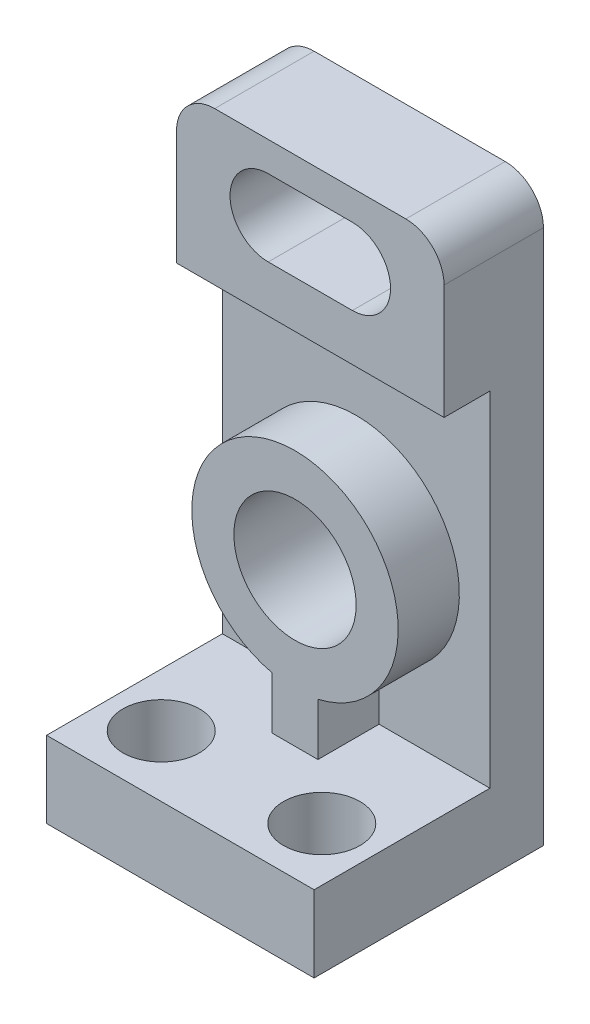
ISO-10303-21;
HEADER;
FILE_DESCRIPTION(('STEP AP214'),'2;1');
FILE_NAME('part.step','',(''),(''),'','','');
FILE_SCHEMA(('AUTOMOTIVE_DESIGN { 1 0 10303 214 1 1 1 1 }'));
ENDSEC;
DATA;
#1=APPLICATION_CONTEXT('core data for automotive mechanical design processes');
#2=APPLICATION_PROTOCOL_DEFINITION('international standard','automotive_design',2000,#1);
#3=PRODUCT_CONTEXT('',#1,'mechanical');
#4=PRODUCT('Part','Part','',(#3));
#5=PRODUCT_RELATED_PRODUCT_CATEGORY('part','',(#4));
#6=PRODUCT_DEFINITION_FORMATION('','',#4);
#7=PRODUCT_DEFINITION_CONTEXT('part definition',#1,'design');
#8=PRODUCT_DEFINITION('design','',#6,#7);
#9=PRODUCT_DEFINITION_SHAPE('','',#8);
#10=(LENGTH_UNIT() NAMED_UNIT(*) SI_UNIT(.MILLI.,.METRE.));
#11=(NAMED_UNIT(*) PLANE_ANGLE_UNIT() SI_UNIT($,.RADIAN.));
#12=(NAMED_UNIT(*) SI_UNIT($,.STERADIAN.) SOLID_ANGLE_UNIT());
#13=UNCERTAINTY_MEASURE_WITH_UNIT(LENGTH_MEASURE(1.E-05),#10,'distance_accuracy_value','');
#14=(GEOMETRIC_REPRESENTATION_CONTEXT(3) GLOBAL_UNCERTAINTY_ASSIGNED_CONTEXT((#13)) GLOBAL_UNIT_ASSIGNED_CONTEXT((#10,
#11,#12)) REPRESENTATION_CONTEXT('',''));
#15=CARTESIAN_POINT('',(0.,0.,0.));
#16=DIRECTION('',(0.,0.,1.));
#17=DIRECTION('',(1.,0.,0.));
#18=AXIS2_PLACEMENT_3D('',#15,#16,#17);
#19=CARTESIAN_POINT('',(0.,10.,0.));
#20=DIRECTION('',(0.,1.,0.));
#21=DIRECTION('',(0.,0.,1.));
#22=AXIS2_PLACEMENT_3D('',#19,#20,#21);
#23=PLANE('',#22);
#24=CARTESIAN_POINT('',(10.5,10.,7.));
#25=DIRECTION('',(0.,1.,0.));
#26=DIRECTION('',(0.,0.,1.));
#27=AXIS2_PLACEMENT_3D('',#24,#25,#26);
#28=CIRCLE('',#27,5.);
#29=CARTESIAN_POINT('',(10.5,10.,12.));
#30=VERTEX_POINT('',#29);
#31=EDGE_CURVE('E288',#30,#30,#28,.T.);
#32=ORIENTED_EDGE('',*,*,#31,.F.);
#33=EDGE_LOOP('',(#32));
#34=FACE_BOUND('',#33,.T.);
#35=CARTESIAN_POINT('',(-10.5,10.,7.));
#36=DIRECTION('',(0.,1.,0.));
#37=DIRECTION('',(0.,0.,1.));
#38=AXIS2_PLACEMENT_3D('',#35,#36,#37);
#39=CIRCLE('',#38,5.);
#40=CARTESIAN_POINT('',(-10.5,10.,12.));
#41=VERTEX_POINT('',#40);
#42=EDGE_CURVE('E619',#41,#41,#39,.T.);
#43=ORIENTED_EDGE('',*,*,#42,.F.);
#44=EDGE_LOOP('',(#43));
#45=FACE_BOUND('',#44,.T.);
#46=DIRECTION('',(1.,0.,0.));
#47=VECTOR('',#46,1.);
#48=CARTESIAN_POINT('',(-17.5,10.,-8.));
#49=LINE('',#48,#47);
#50=CARTESIAN_POINT('',(3.,10.,-8.));
#51=VERTEX_POINT('',#50);
#52=CARTESIAN_POINT('',(17.5,10.,-8.));
#53=VERTEX_POINT('',#52);
#54=EDGE_CURVE('E193',#51,#53,#49,.T.);
#55=ORIENTED_EDGE('',*,*,#54,.F.);
#56=DIRECTION('',(0.,0.,-1.));
#57=VECTOR('',#56,1.);
#58=CARTESIAN_POINT('',(3.,10.,0.));
#59=LINE('',#58,#57);
#60=CARTESIAN_POINT('',(3.,10.,0.));
#61=VERTEX_POINT('',#60);
#62=EDGE_CURVE('E172',#61,#51,#59,.T.);
#63=ORIENTED_EDGE('',*,*,#62,.F.);
#64=DIRECTION('',(1.,0.,0.));
#65=VECTOR('',#64,1.);
#66=CARTESIAN_POINT('',(-3.,10.,0.));
#67=LINE('',#66,#65);
#68=CARTESIAN_POINT('',(-3.,10.,0.));
#69=VERTEX_POINT('',#68);
#70=EDGE_CURVE('E181',#69,#61,#67,.T.);
#71=ORIENTED_EDGE('',*,*,#70,.F.);
#72=DIRECTION('',(0.,0.,-1.));
#73=VECTOR('',#72,1.);
#74=CARTESIAN_POINT('',(-3.,10.,0.));
#75=LINE('',#74,#73);
#76=CARTESIAN_POINT('',(-3.,10.,-8.));
#77=VERTEX_POINT('',#76);
#78=EDGE_CURVE('E632',#69,#77,#75,.T.);
#79=ORIENTED_EDGE('',*,*,#78,.T.);
#80=CARTESIAN_POINT('',(-17.5,10.,-8.));
#81=VERTEX_POINT('',#80);
#82=EDGE_CURVE('E252',#81,#77,#49,.T.);
#83=ORIENTED_EDGE('',*,*,#82,.F.);
#84=DIRECTION('',(0.,0.,1.));
#85=VECTOR('',#84,1.);
#86=CARTESIAN_POINT('',(-17.5,10.,-15.));
#87=LINE('',#86,#85);
#88=CARTESIAN_POINT('',(-17.5,10.,15.));
#89=VERTEX_POINT('',#88);
#90=EDGE_CURVE('E263',#81,#89,#87,.T.);
#91=ORIENTED_EDGE('',*,*,#90,.T.);
#92=DIRECTION('',(1.,0.,0.));
#93=VECTOR('',#92,1.);
#94=CARTESIAN_POINT('',(-17.5,10.,15.));
#95=LINE('',#94,#93);
#96=CARTESIAN_POINT('',(17.5,10.,15.));
#97=VERTEX_POINT('',#96);
#98=EDGE_CURVE('E264',#89,#97,#95,.T.);
#99=ORIENTED_EDGE('',*,*,#98,.T.);
#100=DIRECTION('',(0.,0.,-1.));
#101=VECTOR('',#100,1.);
#102=CARTESIAN_POINT('',(17.5,10.,-15.));
#103=LINE('',#102,#101);
#104=EDGE_CURVE('E256',#97,#53,#103,.T.);
#105=ORIENTED_EDGE('',*,*,#104,.T.);
#106=EDGE_LOOP('',(#55,#63,#71,#79,#83,#91,#99,#105));
#107=FACE_BOUND('',#106,.T.);
#108=ADVANCED_FACE('F50',(#34,#45,#107),#23,.T.);
#109=CARTESIAN_POINT('',(-17.5,75.,-8.));
#110=DIRECTION('',(0.,0.,-1.));
#111=DIRECTION('',(-1.,0.,0.));
#112=AXIS2_PLACEMENT_3D('',#109,#110,#111);
#113=PLANE('',#112);
#114=DIRECTION('',(0.,1.,0.));
#115=VECTOR('',#114,1.);
#116=CARTESIAN_POINT('',(3.,16.8375534189118,-8.));
#117=LINE('',#116,#115);
#118=CARTESIAN_POINT('',(3.,16.8375534189118,-8.));
#119=VERTEX_POINT('',#118);
#120=EDGE_CURVE('E629',#51,#119,#117,.T.);
#121=ORIENTED_EDGE('',*,*,#120,.F.);
#122=ORIENTED_EDGE('',*,*,#54,.T.);
#123=DIRECTION('',(0.,-1.,0.));
#124=VECTOR('',#123,1.);
#125=CARTESIAN_POINT('',(17.5,75.,-8.));
#126=LINE('',#125,#124);
#127=CARTESIAN_POINT('',(17.5,55.,-8.));
#128=VERTEX_POINT('',#127);
#129=EDGE_CURVE('E249',#128,#53,#126,.T.);
#130=ORIENTED_EDGE('',*,*,#129,.F.);
#131=DIRECTION('',(1.,0.,0.));
#132=VECTOR('',#131,1.);
#133=CARTESIAN_POINT('',(-17.5,55.,-8.));
#134=LINE('',#133,#132);
#135=CARTESIAN_POINT('',(-17.5,55.,-8.));
#136=VERTEX_POINT('',#135);
#137=EDGE_CURVE('E227',#136,#128,#134,.T.);
#138=ORIENTED_EDGE('',*,*,#137,.F.);
#139=DIRECTION('',(0.,-1.,0.));
#140=VECTOR('',#139,1.);
#141=CARTESIAN_POINT('',(-17.5,75.,-8.));
#142=LINE('',#141,#140);
#143=EDGE_CURVE('E257',#136,#81,#142,.T.);
#144=ORIENTED_EDGE('',*,*,#143,.T.);
#145=ORIENTED_EDGE('',*,*,#82,.T.);
#146=DIRECTION('',(0.,-1.,0.));
#147=VECTOR('',#146,1.);
#148=CARTESIAN_POINT('',(-3.,16.8375534189118,-8.));
#149=LINE('',#148,#147);
#150=CARTESIAN_POINT('',(-3.,16.8375534189118,-8.));
#151=VERTEX_POINT('',#150);
#152=EDGE_CURVE('E192',#151,#77,#149,.T.);
#153=ORIENTED_EDGE('',*,*,#152,.F.);
#154=CARTESIAN_POINT('',(0.,30.,-8.));
#155=DIRECTION('',(0.,0.,1.));
#156=DIRECTION('',(1.,0.,0.));
#157=AXIS2_PLACEMENT_3D('',#154,#155,#156);
#158=CIRCLE('',#157,13.5);
#159=EDGE_CURVE('E636',#119,#151,#158,.T.);
#160=ORIENTED_EDGE('',*,*,#159,.F.);
#161=EDGE_LOOP('',(#121,#122,#130,#138,#144,#145,#153,#160));
#162=FACE_BOUND('',#161,.T.);
#163=ADVANCED_FACE('F327',(#162),#113,.F.);
#164=CARTESIAN_POINT('',(17.5,10.,-15.));
#165=DIRECTION('',(-1.,0.,0.));
#166=DIRECTION('',(0.,0.,1.));
#167=AXIS2_PLACEMENT_3D('',#164,#165,#166);
#168=PLANE('',#167);
#169=DIRECTION('',(0.,-1.,0.));
#170=VECTOR('',#169,1.);
#171=CARTESIAN_POINT('',(17.5,10.,-15.));
#172=LINE('',#171,#170);
#173=CARTESIAN_POINT('',(17.5,70.,-15.));
#174=VERTEX_POINT('',#173);
#175=CARTESIAN_POINT('',(17.5,0.,-15.));
#176=VERTEX_POINT('',#175);
#177=EDGE_CURVE('E285',#174,#176,#172,.T.);
#178=ORIENTED_EDGE('',*,*,#177,.F.);
#179=DIRECTION('',(0.,0.,-1.));
#180=VECTOR('',#179,1.);
#181=CARTESIAN_POINT('',(17.5,70.,-2.));
#182=LINE('',#181,#180);
#183=CARTESIAN_POINT('',(17.5,70.,-2.));
#184=VERTEX_POINT('',#183);
#185=EDGE_CURVE('E54',#174,#184,#182,.F.);
#186=ORIENTED_EDGE('',*,*,#185,.T.);
#187=DIRECTION('',(0.,1.,0.));
#188=VECTOR('',#187,1.);
#189=CARTESIAN_POINT('',(17.5,55.,-2.));
#190=LINE('',#189,#188);
#191=CARTESIAN_POINT('',(17.5,55.,-2.));
#192=VERTEX_POINT('',#191);
#193=EDGE_CURVE('E238',#192,#184,#190,.T.);
#194=ORIENTED_EDGE('',*,*,#193,.F.);
#195=DIRECTION('',(0.,0.,-1.));
#196=VECTOR('',#195,1.);
#197=CARTESIAN_POINT('',(17.5,55.,-2.));
#198=LINE('',#197,#196);
#199=EDGE_CURVE('E245',#192,#128,#198,.T.);
#200=ORIENTED_EDGE('',*,*,#199,.T.);
#201=ORIENTED_EDGE('',*,*,#129,.T.);
#202=ORIENTED_EDGE('',*,*,#104,.F.);
#203=DIRECTION('',(0.,-1.,0.));
#204=VECTOR('',#203,1.);
#205=CARTESIAN_POINT('',(17.5,10.,15.));
#206=LINE('',#205,#204);
#207=CARTESIAN_POINT('',(17.5,0.,15.));
#208=VERTEX_POINT('',#207);
#209=EDGE_CURVE('E266',#97,#208,#206,.T.);
#210=ORIENTED_EDGE('',*,*,#209,.T.);
#211=DIRECTION('',(0.,0.,-1.));
#212=VECTOR('',#211,1.);
#213=CARTESIAN_POINT('',(17.5,0.,-15.));
#214=LINE('',#213,#212);
#215=EDGE_CURVE('E259',#208,#176,#214,.T.);
#216=ORIENTED_EDGE('',*,*,#215,.T.);
#217=EDGE_LOOP('',(#178,#186,#194,#200,#201,#202,#210,#216));
#218=FACE_BOUND('',#217,.T.);
#219=ADVANCED_FACE('F333',(#218),#168,.F.);
#220=CARTESIAN_POINT('',(-17.5,10.,-15.));
#221=DIRECTION('',(0.,0.,1.));
#222=DIRECTION('',(1.,0.,0.));
#223=AXIS2_PLACEMENT_3D('',#220,#221,#222);
#224=PLANE('',#223);
#225=CARTESIAN_POINT('',(0.,30.,-15.));
#226=DIRECTION('',(0.,0.,1.));
#227=DIRECTION('',(1.,0.,0.));
#228=AXIS2_PLACEMENT_3D('',#225,#226,#227);
#229=CIRCLE('',#228,8.);
#230=CARTESIAN_POINT('',(8.,30.,-15.));
#231=VERTEX_POINT('',#230);
#232=EDGE_CURVE('E282',#231,#231,#229,.T.);
#233=ORIENTED_EDGE('',*,*,#232,.T.);
#234=EDGE_LOOP('',(#233));
#235=FACE_BOUND('',#234,.T.);
#236=DIRECTION('',(-1.,0.,0.));
#237=VECTOR('',#236,1.);
#238=CARTESIAN_POINT('',(-5.49999999999999,71.1249870936973,-15.));
#239=LINE('',#238,#237);
#240=CARTESIAN_POINT('',(5.49999999999999,71.1249870936973,-15.));
#241=VERTEX_POINT('',#240);
#242=CARTESIAN_POINT('',(-5.49999999999999,71.1249870936973,-15.));
#243=VERTEX_POINT('',#242);
#244=EDGE_CURVE('E211',#241,#243,#239,.T.);
#245=ORIENTED_EDGE('',*,*,#244,.T.);
#246=CARTESIAN_POINT('',(-5.49999999999999,66.1249870936973,-15.));
#247=DIRECTION('',(0.,0.,1.));
#248=DIRECTION('',(1.,0.,0.));
#249=AXIS2_PLACEMENT_3D('',#246,#247,#248);
#250=CIRCLE('',#249,5.);
#251=CARTESIAN_POINT('',(-5.49999999999999,61.1249870936973,-15.));
#252=VERTEX_POINT('',#251);
#253=EDGE_CURVE('E202',#243,#252,#250,.T.);
#254=ORIENTED_EDGE('',*,*,#253,.T.);
#255=DIRECTION('',(1.,0.,0.));
#256=VECTOR('',#255,1.);
#257=CARTESIAN_POINT('',(-5.49999999999999,61.1249870936973,-15.));
#258=LINE('',#257,#256);
#259=CARTESIAN_POINT('',(5.49999999999999,61.1249870936973,-15.));
#260=VERTEX_POINT('',#259);
#261=EDGE_CURVE('E210',#252,#260,#258,.T.);
#262=ORIENTED_EDGE('',*,*,#261,.T.);
#263=CARTESIAN_POINT('',(5.50000000000001,66.1249870936973,-15.));
#264=DIRECTION('',(0.,0.,1.));
#265=DIRECTION('',(1.,0.,0.));
#266=AXIS2_PLACEMENT_3D('',#263,#264,#265);
#267=CIRCLE('',#266,5.);
#268=EDGE_CURVE('E212',#260,#241,#267,.T.);
#269=ORIENTED_EDGE('',*,*,#268,.T.);
#270=EDGE_LOOP('',(#245,#254,#262,#269));
#271=FACE_BOUND('',#270,.T.);
#272=DIRECTION('',(-1.,0.,0.));
#273=VECTOR('',#272,1.);
#274=CARTESIAN_POINT('',(17.5,75.,-15.));
#275=LINE('',#274,#273);
#276=CARTESIAN_POINT('',(12.5,75.,-15.));
#277=VERTEX_POINT('',#276);
#278=CARTESIAN_POINT('',(-12.5,75.,-15.));
#279=VERTEX_POINT('',#278);
#280=EDGE_CURVE('E247',#277,#279,#275,.T.);
#281=ORIENTED_EDGE('',*,*,#280,.F.);
#282=CARTESIAN_POINT('',(12.5,70.,-15.));
#283=DIRECTION('',(0.,0.,1.));
#284=DIRECTION('',(1.,0.,0.));
#285=AXIS2_PLACEMENT_3D('',#282,#283,#284);
#286=CIRCLE('',#285,5.);
#287=EDGE_CURVE('E69',#277,#174,#286,.F.);
#288=ORIENTED_EDGE('',*,*,#287,.T.);
#289=ORIENTED_EDGE('',*,*,#177,.T.);
#290=DIRECTION('',(-1.,0.,0.));
#291=VECTOR('',#290,1.);
#292=CARTESIAN_POINT('',(-17.5,0.,-15.));
#293=LINE('',#292,#291);
#294=CARTESIAN_POINT('',(-17.5,0.,-15.));
#295=VERTEX_POINT('',#294);
#296=EDGE_CURVE('E267',#176,#295,#293,.T.);
#297=ORIENTED_EDGE('',*,*,#296,.T.);
#298=DIRECTION('',(0.,-1.,0.));
#299=VECTOR('',#298,1.);
#300=CARTESIAN_POINT('',(-17.5,10.,-15.));
#301=LINE('',#300,#299);
#302=CARTESIAN_POINT('',(-17.5,70.,-15.));
#303=VERTEX_POINT('',#302);
#304=EDGE_CURVE('E278',#303,#295,#301,.T.);
#305=ORIENTED_EDGE('',*,*,#304,.F.);
#306=CARTESIAN_POINT('',(-12.5,70.,-15.));
#307=DIRECTION('',(0.,0.,1.));
#308=DIRECTION('',(1.,0.,0.));
#309=AXIS2_PLACEMENT_3D('',#306,#307,#308);
#310=CIRCLE('',#309,5.);
#311=EDGE_CURVE('E294',#303,#279,#310,.F.);
#312=ORIENTED_EDGE('',*,*,#311,.T.);
#313=EDGE_LOOP('',(#281,#288,#289,#297,#305,#312));
#314=FACE_BOUND('',#313,.T.);
#315=ADVANCED_FACE('F310',(#235,#271,#314),#224,.F.);
#316=CARTESIAN_POINT('',(-17.5,10.,-15.));
#317=DIRECTION('',(1.,0.,0.));
#318=DIRECTION('',(0.,0.,-1.));
#319=AXIS2_PLACEMENT_3D('',#316,#317,#318);
#320=PLANE('',#319);
#321=DIRECTION('',(0.,-1.,0.));
#322=VECTOR('',#321,1.);
#323=CARTESIAN_POINT('',(-17.5,75.,-2.));
#324=LINE('',#323,#322);
#325=CARTESIAN_POINT('',(-17.5,70.,-2.));
#326=VERTEX_POINT('',#325);
#327=CARTESIAN_POINT('',(-17.5,55.,-2.));
#328=VERTEX_POINT('',#327);
#329=EDGE_CURVE('E234',#326,#328,#324,.T.);
#330=ORIENTED_EDGE('',*,*,#329,.F.);
#331=DIRECTION('',(0.,0.,1.));
#332=VECTOR('',#331,1.);
#333=CARTESIAN_POINT('',(-17.5,70.,-15.));
#334=LINE('',#333,#332);
#335=EDGE_CURVE('E291',#326,#303,#334,.F.);
#336=ORIENTED_EDGE('',*,*,#335,.T.);
#337=ORIENTED_EDGE('',*,*,#304,.T.);
#338=DIRECTION('',(0.,0.,1.));
#339=VECTOR('',#338,1.);
#340=CARTESIAN_POINT('',(-17.5,0.,-15.));
#341=LINE('',#340,#339);
#342=CARTESIAN_POINT('',(-17.5,0.,15.));
#343=VERTEX_POINT('',#342);
#344=EDGE_CURVE('E275',#295,#343,#341,.T.);
#345=ORIENTED_EDGE('',*,*,#344,.T.);
#346=DIRECTION('',(0.,-1.,0.));
#347=VECTOR('',#346,1.);
#348=CARTESIAN_POINT('',(-17.5,10.,15.));
#349=LINE('',#348,#347);
#350=EDGE_CURVE('E280',#89,#343,#349,.T.);
#351=ORIENTED_EDGE('',*,*,#350,.F.);
#352=ORIENTED_EDGE('',*,*,#90,.F.);
#353=ORIENTED_EDGE('',*,*,#143,.F.);
#354=DIRECTION('',(0.,0.,-1.));
#355=VECTOR('',#354,1.);
#356=CARTESIAN_POINT('',(-17.5,55.,-2.));
#357=LINE('',#356,#355);
#358=EDGE_CURVE('E246',#328,#136,#357,.T.);
#359=ORIENTED_EDGE('',*,*,#358,.F.);
#360=EDGE_LOOP('',(#330,#336,#337,#345,#351,#352,#353,#359));
#361=FACE_BOUND('',#360,.T.);
#362=ADVANCED_FACE('F322',(#361),#320,.F.);
#363=CARTESIAN_POINT('',(-17.5,10.,15.));
#364=DIRECTION('',(0.,0.,-1.));
#365=DIRECTION('',(-1.,0.,0.));
#366=AXIS2_PLACEMENT_3D('',#363,#364,#365);
#367=PLANE('',#366);
#368=DIRECTION('',(1.,0.,0.));
#369=VECTOR('',#368,1.);
#370=CARTESIAN_POINT('',(-17.5,0.,15.));
#371=LINE('',#370,#369);
#372=EDGE_CURVE('E265',#343,#208,#371,.T.);
#373=ORIENTED_EDGE('',*,*,#372,.T.);
#374=ORIENTED_EDGE('',*,*,#209,.F.);
#375=ORIENTED_EDGE('',*,*,#98,.F.);
#376=ORIENTED_EDGE('',*,*,#350,.T.);
#377=EDGE_LOOP('',(#373,#374,#375,#376));
#378=FACE_BOUND('',#377,.T.);
#379=ADVANCED_FACE('F336',(#378),#367,.F.);
#380=CARTESIAN_POINT('',(0.,0.,0.));
#381=DIRECTION('',(0.,1.,0.));
#382=DIRECTION('',(0.,0.,1.));
#383=AXIS2_PLACEMENT_3D('',#380,#381,#382);
#384=PLANE('',#383);
#385=CARTESIAN_POINT('',(10.5,0.,7.));
#386=DIRECTION('',(0.,1.,0.));
#387=DIRECTION('',(0.,0.,1.));
#388=AXIS2_PLACEMENT_3D('',#385,#386,#387);
#389=CIRCLE('',#388,5.);
#390=CARTESIAN_POINT('',(10.5,0.,12.));
#391=VERTEX_POINT('',#390);
#392=EDGE_CURVE('E617',#391,#391,#389,.T.);
#393=ORIENTED_EDGE('',*,*,#392,.T.);
#394=EDGE_LOOP('',(#393));
#395=FACE_BOUND('',#394,.T.);
#396=CARTESIAN_POINT('',(-10.5,0.,7.));
#397=DIRECTION('',(0.,1.,0.));
#398=DIRECTION('',(0.,0.,1.));
#399=AXIS2_PLACEMENT_3D('',#396,#397,#398);
#400=CIRCLE('',#399,5.);
#401=CARTESIAN_POINT('',(-10.5,0.,12.));
#402=VERTEX_POINT('',#401);
#403=EDGE_CURVE('E621',#402,#402,#400,.T.);
#404=ORIENTED_EDGE('',*,*,#403,.T.);
#405=EDGE_LOOP('',(#404));
#406=FACE_BOUND('',#405,.T.);
#407=ORIENTED_EDGE('',*,*,#215,.F.);
#408=ORIENTED_EDGE('',*,*,#372,.F.);
#409=ORIENTED_EDGE('',*,*,#344,.F.);
#410=ORIENTED_EDGE('',*,*,#296,.F.);
#411=EDGE_LOOP('',(#407,#408,#409,#410));
#412=FACE_BOUND('',#411,.T.);
#413=ADVANCED_FACE('F344',(#395,#406,#412),#384,.F.);
#414=CARTESIAN_POINT('',(0.,75.,0.));
#415=DIRECTION('',(0.,1.,0.));
#416=DIRECTION('',(0.,0.,1.));
#417=AXIS2_PLACEMENT_3D('',#414,#415,#416);
#418=PLANE('',#417);
#419=DIRECTION('',(-1.,0.,0.));
#420=VECTOR('',#419,1.);
#421=CARTESIAN_POINT('',(17.5,75.,-2.));
#422=LINE('',#421,#420);
#423=CARTESIAN_POINT('',(12.5,75.,-2.));
#424=VERTEX_POINT('',#423);
#425=CARTESIAN_POINT('',(-12.5,75.,-2.));
#426=VERTEX_POINT('',#425);
#427=EDGE_CURVE('E239',#424,#426,#422,.T.);
#428=ORIENTED_EDGE('',*,*,#427,.F.);
#429=DIRECTION('',(0.,0.,-1.));
#430=VECTOR('',#429,1.);
#431=CARTESIAN_POINT('',(12.5,75.,-15.));
#432=LINE('',#431,#430);
#433=EDGE_CURVE('E296',#424,#277,#432,.T.);
#434=ORIENTED_EDGE('',*,*,#433,.T.);
#435=ORIENTED_EDGE('',*,*,#280,.T.);
#436=DIRECTION('',(0.,0.,1.));
#437=VECTOR('',#436,1.);
#438=CARTESIAN_POINT('',(-12.5,75.,-2.));
#439=LINE('',#438,#437);
#440=EDGE_CURVE('E284',#279,#426,#439,.T.);
#441=ORIENTED_EDGE('',*,*,#440,.T.);
#442=EDGE_LOOP('',(#428,#434,#435,#441));
#443=FACE_BOUND('',#442,.T.);
#444=ADVANCED_FACE('F302',(#443),#418,.T.);
#445=CARTESIAN_POINT('',(-17.5,55.,-2.));
#446=DIRECTION('',(0.,1.,0.));
#447=DIRECTION('',(0.,0.,1.));
#448=AXIS2_PLACEMENT_3D('',#445,#446,#447);
#449=PLANE('',#448);
#450=ORIENTED_EDGE('',*,*,#137,.T.);
#451=ORIENTED_EDGE('',*,*,#199,.F.);
#452=DIRECTION('',(1.,0.,0.));
#453=VECTOR('',#452,1.);
#454=CARTESIAN_POINT('',(-17.5,55.,-2.));
#455=LINE('',#454,#453);
#456=EDGE_CURVE('E236',#328,#192,#455,.T.);
#457=ORIENTED_EDGE('',*,*,#456,.F.);
#458=ORIENTED_EDGE('',*,*,#358,.T.);
#459=EDGE_LOOP('',(#450,#451,#457,#458));
#460=FACE_BOUND('',#459,.T.);
#461=ADVANCED_FACE('F328',(#460),#449,.F.);
#462=CARTESIAN_POINT('',(0.,0.,-2.));
#463=DIRECTION('',(0.,0.,1.));
#464=DIRECTION('',(1.,0.,0.));
#465=AXIS2_PLACEMENT_3D('',#462,#463,#464);
#466=PLANE('',#465);
#467=CARTESIAN_POINT('',(-5.49999999999999,66.1249870936973,-2.));
#468=DIRECTION('',(0.,0.,1.));
#469=DIRECTION('',(1.,0.,0.));
#470=AXIS2_PLACEMENT_3D('',#467,#468,#469);
#471=CIRCLE('',#470,5.);
#472=CARTESIAN_POINT('',(-5.49999999999999,71.1249870936973,-2.));
#473=VERTEX_POINT('',#472);
#474=CARTESIAN_POINT('',(-5.49999999999999,61.1249870936973,-2.));
#475=VERTEX_POINT('',#474);
#476=EDGE_CURVE('E198',#473,#475,#471,.T.);
#477=ORIENTED_EDGE('',*,*,#476,.F.);
#478=DIRECTION('',(-1.,0.,0.));
#479=VECTOR('',#478,1.);
#480=CARTESIAN_POINT('',(-5.49999999999999,71.1249870936973,-2.));
#481=LINE('',#480,#479);
#482=CARTESIAN_POINT('',(5.49999999999999,71.1249870936973,-2.));
#483=VERTEX_POINT('',#482);
#484=EDGE_CURVE('E206',#483,#473,#481,.T.);
#485=ORIENTED_EDGE('',*,*,#484,.F.);
#486=CARTESIAN_POINT('',(5.50000000000001,66.1249870936973,-2.));
#487=DIRECTION('',(0.,0.,1.));
#488=DIRECTION('',(1.,0.,0.));
#489=AXIS2_PLACEMENT_3D('',#486,#487,#488);
#490=CIRCLE('',#489,5.);
#491=CARTESIAN_POINT('',(5.49999999999999,61.1249870936973,-2.));
#492=VERTEX_POINT('',#491);
#493=EDGE_CURVE('E217',#492,#483,#490,.T.);
#494=ORIENTED_EDGE('',*,*,#493,.F.);
#495=DIRECTION('',(1.,0.,0.));
#496=VECTOR('',#495,1.);
#497=CARTESIAN_POINT('',(-5.49999999999999,61.1249870936973,-2.));
#498=LINE('',#497,#496);
#499=EDGE_CURVE('E196',#475,#492,#498,.T.);
#500=ORIENTED_EDGE('',*,*,#499,.F.);
#501=EDGE_LOOP('',(#477,#485,#494,#500));
#502=FACE_BOUND('',#501,.T.);
#503=ORIENTED_EDGE('',*,*,#193,.T.);
#504=CARTESIAN_POINT('',(12.5,70.,-2.));
#505=DIRECTION('',(0.,0.,1.));
#506=DIRECTION('',(1.,0.,0.));
#507=AXIS2_PLACEMENT_3D('',#504,#505,#506);
#508=CIRCLE('',#507,5.);
#509=EDGE_CURVE('E11',#184,#424,#508,.T.);
#510=ORIENTED_EDGE('',*,*,#509,.T.);
#511=ORIENTED_EDGE('',*,*,#427,.T.);
#512=CARTESIAN_POINT('',(-12.5,70.,-2.));
#513=DIRECTION('',(0.,0.,1.));
#514=DIRECTION('',(1.,0.,0.));
#515=AXIS2_PLACEMENT_3D('',#512,#513,#514);
#516=CIRCLE('',#515,5.);
#517=EDGE_CURVE('E293',#426,#326,#516,.T.);
#518=ORIENTED_EDGE('',*,*,#517,.T.);
#519=ORIENTED_EDGE('',*,*,#329,.T.);
#520=ORIENTED_EDGE('',*,*,#456,.T.);
#521=EDGE_LOOP('',(#503,#510,#511,#518,#519,#520));
#522=FACE_BOUND('',#521,.T.);
#523=ADVANCED_FACE('F320',(#502,#522),#466,.T.);
#524=CARTESIAN_POINT('',(-5.49999999999999,66.1249870936973,-15.));
#525=DIRECTION('',(0.,0.,1.));
#526=DIRECTION('',(1.,0.,0.));
#527=AXIS2_PLACEMENT_3D('',#524,#525,#526);
#528=CYLINDRICAL_SURFACE('',#527,5.);
#529=ORIENTED_EDGE('',*,*,#476,.T.);
#530=DIRECTION('',(0.,0.,1.));
#531=VECTOR('',#530,1.);
#532=CARTESIAN_POINT('',(-5.49999999999999,61.1249870936973,-15.));
#533=LINE('',#532,#531);
#534=EDGE_CURVE('E218',#252,#475,#533,.T.);
#535=ORIENTED_EDGE('',*,*,#534,.F.);
#536=ORIENTED_EDGE('',*,*,#253,.F.);
#537=DIRECTION('',(0.,0.,1.));
#538=VECTOR('',#537,1.);
#539=CARTESIAN_POINT('',(-5.49999999999999,71.1249870936973,-15.));
#540=LINE('',#539,#538);
#541=EDGE_CURVE('E224',#243,#473,#540,.T.);
#542=ORIENTED_EDGE('',*,*,#541,.T.);
#543=EDGE_LOOP('',(#529,#535,#536,#542));
#544=FACE_BOUND('',#543,.T.);
#545=ADVANCED_FACE('F398',(#544),#528,.F.);
#546=CARTESIAN_POINT('',(-5.49999999999999,71.1249870936973,-15.));
#547=DIRECTION('',(0.,1.,0.));
#548=DIRECTION('',(0.,0.,1.));
#549=AXIS2_PLACEMENT_3D('',#546,#547,#548);
#550=PLANE('',#549);
#551=ORIENTED_EDGE('',*,*,#484,.T.);
#552=ORIENTED_EDGE('',*,*,#541,.F.);
#553=ORIENTED_EDGE('',*,*,#244,.F.);
#554=DIRECTION('',(0.,0.,1.));
#555=VECTOR('',#554,1.);
#556=CARTESIAN_POINT('',(5.49999999999999,71.1249870936973,-15.));
#557=LINE('',#556,#555);
#558=EDGE_CURVE('E226',#241,#483,#557,.T.);
#559=ORIENTED_EDGE('',*,*,#558,.T.);
#560=EDGE_LOOP('',(#551,#552,#553,#559));
#561=FACE_BOUND('',#560,.T.);
#562=ADVANCED_FACE('F416',(#561),#550,.F.);
#563=CARTESIAN_POINT('',(5.50000000000001,66.1249870936973,-15.));
#564=DIRECTION('',(0.,0.,1.));
#565=DIRECTION('',(1.,0.,0.));
#566=AXIS2_PLACEMENT_3D('',#563,#564,#565);
#567=CYLINDRICAL_SURFACE('',#566,5.);
#568=ORIENTED_EDGE('',*,*,#493,.T.);
#569=ORIENTED_EDGE('',*,*,#558,.F.);
#570=ORIENTED_EDGE('',*,*,#268,.F.);
#571=DIRECTION('',(0.,0.,1.));
#572=VECTOR('',#571,1.);
#573=CARTESIAN_POINT('',(5.49999999999999,61.1249870936973,-15.));
#574=LINE('',#573,#572);
#575=EDGE_CURVE('E229',#260,#492,#574,.T.);
#576=ORIENTED_EDGE('',*,*,#575,.T.);
#577=EDGE_LOOP('',(#568,#569,#570,#576));
#578=FACE_BOUND('',#577,.T.);
#579=ADVANCED_FACE('F426',(#578),#567,.F.);
#580=CARTESIAN_POINT('',(-5.49999999999999,61.1249870936973,-15.));
#581=DIRECTION('',(0.,-1.,0.));
#582=DIRECTION('',(0.,0.,-1.));
#583=AXIS2_PLACEMENT_3D('',#580,#581,#582);
#584=PLANE('',#583);
#585=ORIENTED_EDGE('',*,*,#499,.T.);
#586=ORIENTED_EDGE('',*,*,#575,.F.);
#587=ORIENTED_EDGE('',*,*,#261,.F.);
#588=ORIENTED_EDGE('',*,*,#534,.T.);
#589=EDGE_LOOP('',(#585,#586,#587,#588));
#590=FACE_BOUND('',#589,.T.);
#591=ADVANCED_FACE('F439',(#590),#584,.F.);
#592=CARTESIAN_POINT('',(0.,30.,0.));
#593=DIRECTION('',(0.,0.,1.));
#594=DIRECTION('',(1.,0.,0.));
#595=AXIS2_PLACEMENT_3D('',#592,#593,#594);
#596=PLANE('',#595);
#597=ORIENTED_EDGE('',*,*,#70,.T.);
#598=DIRECTION('',(0.,1.,0.));
#599=VECTOR('',#598,1.);
#600=CARTESIAN_POINT('',(3.,16.8375534189118,0.));
#601=LINE('',#600,#599);
#602=CARTESIAN_POINT('',(3.,16.8375534189118,0.));
#603=VERTEX_POINT('',#602);
#604=EDGE_CURVE('E167',#61,#603,#601,.T.);
#605=ORIENTED_EDGE('',*,*,#604,.T.);
#606=CARTESIAN_POINT('',(0.,30.,0.));
#607=DIRECTION('',(0.,0.,1.));
#608=DIRECTION('',(1.,0.,0.));
#609=AXIS2_PLACEMENT_3D('',#606,#607,#608);
#610=CIRCLE('',#609,13.5);
#611=CARTESIAN_POINT('',(-3.,16.8375534189118,0.));
#612=VERTEX_POINT('',#611);
#613=EDGE_CURVE('E179',#603,#612,#610,.T.);
#614=ORIENTED_EDGE('',*,*,#613,.T.);
#615=DIRECTION('',(0.,-1.,0.));
#616=VECTOR('',#615,1.);
#617=CARTESIAN_POINT('',(-3.,16.8375534189118,0.));
#618=LINE('',#617,#616);
#619=EDGE_CURVE('E190',#612,#69,#618,.T.);
#620=ORIENTED_EDGE('',*,*,#619,.T.);
#621=EDGE_LOOP('',(#597,#605,#614,#620));
#622=FACE_BOUND('',#621,.T.);
#623=CARTESIAN_POINT('',(0.,30.,0.));
#624=DIRECTION('',(0.,0.,1.));
#625=DIRECTION('',(1.,0.,0.));
#626=AXIS2_PLACEMENT_3D('',#623,#624,#625);
#627=CIRCLE('',#626,8.);
#628=CARTESIAN_POINT('',(8.,30.,0.));
#629=VERTEX_POINT('',#628);
#630=EDGE_CURVE('E626',#629,#629,#627,.T.);
#631=ORIENTED_EDGE('',*,*,#630,.F.);
#632=EDGE_LOOP('',(#631));
#633=FACE_BOUND('',#632,.T.);
#634=ADVANCED_FACE('F183',(#622,#633),#596,.T.);
#635=CARTESIAN_POINT('',(3.,16.8375534189118,0.));
#636=DIRECTION('',(-1.,0.,0.));
#637=DIRECTION('',(0.,0.,1.));
#638=AXIS2_PLACEMENT_3D('',#635,#636,#637);
#639=PLANE('',#638);
#640=ORIENTED_EDGE('',*,*,#120,.T.);
#641=DIRECTION('',(0.,0.,-1.));
#642=VECTOR('',#641,1.);
#643=CARTESIAN_POINT('',(3.,16.8375534189118,0.));
#644=LINE('',#643,#642);
#645=EDGE_CURVE('E180',#603,#119,#644,.T.);
#646=ORIENTED_EDGE('',*,*,#645,.F.);
#647=ORIENTED_EDGE('',*,*,#604,.F.);
#648=ORIENTED_EDGE('',*,*,#62,.T.);
#649=EDGE_LOOP('',(#640,#646,#647,#648));
#650=FACE_BOUND('',#649,.T.);
#651=ADVANCED_FACE('F175',(#650),#639,.F.);
#652=CARTESIAN_POINT('',(0.,30.,0.));
#653=DIRECTION('',(0.,0.,-1.));
#654=DIRECTION('',(-1.,0.,0.));
#655=AXIS2_PLACEMENT_3D('',#652,#653,#654);
#656=CYLINDRICAL_SURFACE('',#655,13.5);
#657=ORIENTED_EDGE('',*,*,#159,.T.);
#658=DIRECTION('',(0.,0.,-1.));
#659=VECTOR('',#658,1.);
#660=CARTESIAN_POINT('',(-3.,16.8375534189118,0.));
#661=LINE('',#660,#659);
#662=EDGE_CURVE('E197',#612,#151,#661,.T.);
#663=ORIENTED_EDGE('',*,*,#662,.F.);
#664=ORIENTED_EDGE('',*,*,#613,.F.);
#665=ORIENTED_EDGE('',*,*,#645,.T.);
#666=EDGE_LOOP('',(#657,#663,#664,#665));
#667=FACE_BOUND('',#666,.T.);
#668=ADVANCED_FACE('F471',(#667),#656,.T.);
#669=CARTESIAN_POINT('',(-3.,16.8375534189118,0.));
#670=DIRECTION('',(1.,0.,0.));
#671=DIRECTION('',(0.,0.,-1.));
#672=AXIS2_PLACEMENT_3D('',#669,#670,#671);
#673=PLANE('',#672);
#674=ORIENTED_EDGE('',*,*,#152,.T.);
#675=ORIENTED_EDGE('',*,*,#78,.F.);
#676=ORIENTED_EDGE('',*,*,#619,.F.);
#677=ORIENTED_EDGE('',*,*,#662,.T.);
#678=EDGE_LOOP('',(#674,#675,#676,#677));
#679=FACE_BOUND('',#678,.T.);
#680=ADVANCED_FACE('F483',(#679),#673,.F.);
#681=CARTESIAN_POINT('',(0.,30.,0.));
#682=DIRECTION('',(0.,0.,-1.));
#683=DIRECTION('',(-1.,0.,0.));
#684=AXIS2_PLACEMENT_3D('',#681,#682,#683);
#685=CYLINDRICAL_SURFACE('',#684,8.);
#686=ORIENTED_EDGE('',*,*,#630,.T.);
#687=EDGE_LOOP('',(#686));
#688=FACE_BOUND('',#687,.T.);
#689=ORIENTED_EDGE('',*,*,#232,.F.);
#690=EDGE_LOOP('',(#689));
#691=FACE_BOUND('',#690,.T.);
#692=ADVANCED_FACE('F491',(#688,#691),#685,.F.);
#693=CARTESIAN_POINT('',(-10.5,0.,7.));
#694=DIRECTION('',(0.,1.,0.));
#695=DIRECTION('',(0.,0.,1.));
#696=AXIS2_PLACEMENT_3D('',#693,#694,#695);
#697=CYLINDRICAL_SURFACE('',#696,5.);
#698=ORIENTED_EDGE('',*,*,#403,.F.);
#699=EDGE_LOOP('',(#698));
#700=FACE_BOUND('',#699,.T.);
#701=ORIENTED_EDGE('',*,*,#42,.T.);
#702=EDGE_LOOP('',(#701));
#703=FACE_BOUND('',#702,.T.);
#704=ADVANCED_FACE('F502',(#700,#703),#697,.F.);
#705=CARTESIAN_POINT('',(10.5,0.,7.));
#706=DIRECTION('',(0.,1.,0.));
#707=DIRECTION('',(0.,0.,1.));
#708=AXIS2_PLACEMENT_3D('',#705,#706,#707);
#709=CYLINDRICAL_SURFACE('',#708,5.);
#710=ORIENTED_EDGE('',*,*,#392,.F.);
#711=EDGE_LOOP('',(#710));
#712=FACE_BOUND('',#711,.T.);
#713=ORIENTED_EDGE('',*,*,#31,.T.);
#714=EDGE_LOOP('',(#713));
#715=FACE_BOUND('',#714,.T.);
#716=ADVANCED_FACE('F347',(#712,#715),#709,.F.);
#717=CARTESIAN_POINT('',(-12.5,70.,0.));
#718=DIRECTION('',(0.,0.,-1.));
#719=DIRECTION('',(-1.,0.,0.));
#720=AXIS2_PLACEMENT_3D('',#717,#718,#719);
#721=CYLINDRICAL_SURFACE('',#720,5.);
#722=ORIENTED_EDGE('',*,*,#311,.F.);
#723=ORIENTED_EDGE('',*,*,#335,.F.);
#724=ORIENTED_EDGE('',*,*,#517,.F.);
#725=ORIENTED_EDGE('',*,*,#440,.F.);
#726=EDGE_LOOP('',(#722,#723,#724,#725));
#727=FACE_BOUND('',#726,.T.);
#728=ADVANCED_FACE('F313',(#727),#721,.T.);
#729=CARTESIAN_POINT('',(12.5,70.,0.));
#730=DIRECTION('',(0.,0.,1.));
#731=DIRECTION('',(1.,0.,0.));
#732=AXIS2_PLACEMENT_3D('',#729,#730,#731);
#733=CYLINDRICAL_SURFACE('',#732,5.);
#734=ORIENTED_EDGE('',*,*,#509,.F.);
#735=ORIENTED_EDGE('',*,*,#185,.F.);
#736=ORIENTED_EDGE('',*,*,#287,.F.);
#737=ORIENTED_EDGE('',*,*,#433,.F.);
#738=EDGE_LOOP('',(#734,#735,#736,#737));
#739=FACE_BOUND('',#738,.T.);
#740=ADVANCED_FACE('F47',(#739),#733,.T.);
#741=CLOSED_SHELL('',(#108,#163,#219,#315,#362,#379,#413,#444,#461,#523,#545,#562,#579,#591,
#634,#651,#668,#680,#692,#704,#716,#728,#740));
#742=MANIFOLD_SOLID_BREP('B2',#741);
#743=ADVANCED_BREP_SHAPE_REPRESENTATION('',(#18,#742),#14);
#744=SHAPE_DEFINITION_REPRESENTATION(#9,#743);
ENDSEC;
END-ISO-10303-21;
